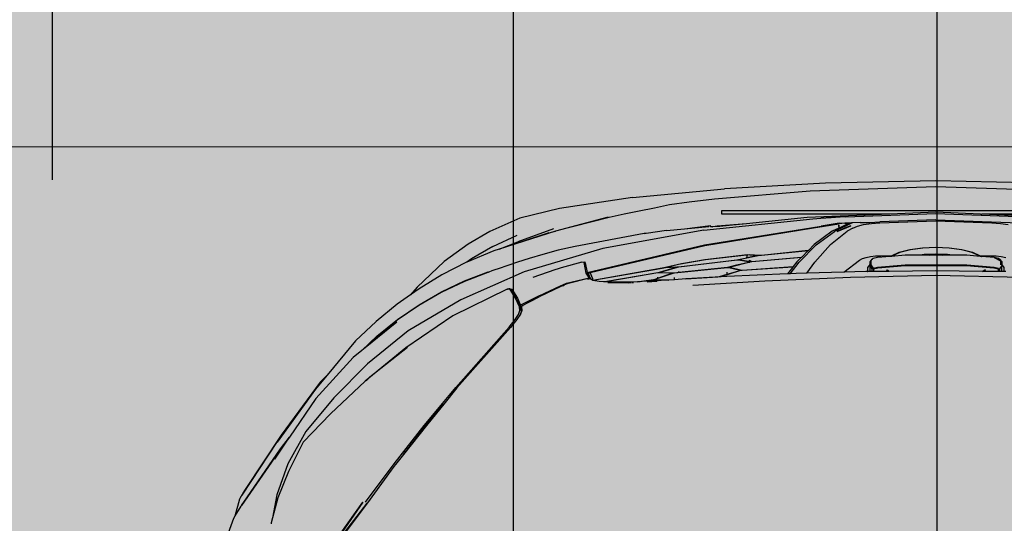
# Model space of a CAD drawing. Units: inches. Extents: x 1884 to 2398, y 474 to 1488.
# Tile 16 of 39: x 2186 to 2233, y 736 to 761. Entities that reach past the tile are written whole.
import ezdxf

# ---------------------------------------------------------------- set-up
doc = ezdxf.new("R2010")
doc.units = ezdxf.units.IN
doc.header["$MEASUREMENT"] = 0
doc.layers.get('0').update_dxf_attribs({"color": 250})
for name, color, linetype, lineweight in [('A-ANNO-DIMS', 2, 'Continuous', 18), ('A-FLOR-STRS', 7, 'Continuous', 20), ('C-VEHI', 8, 'Continuous', 18)]:
    doc.layers.add(name, color=color, linetype=linetype, lineweight=lineweight)
doc.layers.add('A-FLOR-STRS-PATT', color=251, linetype='Continuous', lineweight=13, true_color=0x636466)
doc.layers.add('L-PVMT-PATT', color=9, linetype='Continuous', lineweight=13, true_color=0xc7c8ca)
doc.layers.add('Edges', color=250, linetype='Continuous')
doc.styles.get("Standard").update_dxf_attribs({"font": 'arial.ttf'})
doc.dimstyles.get("Standard").update_dxf_attribs({"dimtxt": 7, "dimasz": 0.18, "dimexe": 0.18, "dimexo": 0.0625, "dimgap": 0.09, "dimtad": 0, "dimtih": 1, "dimtoh": 1, "dimzin": 0, "dimdsep": 46, "dimlunit": 3, "dimtxsty": 'Standard', "dimcen": 0.09, "dimadec": 0, "dimazin": 0, "dimtfac": 1, "dimtofl": 0, "dimtmove": 0, "dimatfit": 3, "dimfxl": 1, "dimtolj": 1, "dimtzin": 0, "dimarcsym": 0})

# ---------------------------------------------------------------- blocks, each defined once
blk = doc.blocks.new('Nissan Qashqai pl')
at = {"layer": 'Edges'}
for p, q in [((7.3216, 11.6621), (7.3216, 12.1821)), ((7.3261, 12.1821), (7.3261, 11.9779)), ((7.298, 12.075), (7.2928, 11.9221)), ((7.3302, 12.0785), (7.3261, 11.9779)), ((7.2884, 12.0562), (7.2857, 11.9221)), ((7.3251, 11.9221), (7.3291, 12.0316)), ((7.3329, 11.9221), (7.3365, 12.0237)), ((7.4002, 11.9221), (7.4025, 12.026)), ((7.3373, 12.0004), (7.3386, 12.01)), ((7.3775, 12.0015), (7.3786, 12.007)), ((7.3909, 12.0051), (7.387, 12.0021)), ((7.3956, 12.0051), (7.3909, 12.0051)), ((7.3959, 12.0049), (7.3956, 12.0051)), ((7.3959, 12.0051), (7.3956, 12.0051)), ((7.3959, 12.0049), (7.3958, 12.0018)), ((7.3959, 12.0071), (7.3959, 12.0051)), ((7.3959, 12.0051), (7.3959, 12.0049)), ((7.3367, 11.99), (7.3373, 12.0004)), ((7.3765, 11.989), (7.3768, 11.9954)), ((7.3768, 11.9954), (7.3775, 12.0015)), ((7.3787, 11.9928), (7.3774, 11.9778)), ((7.3798, 11.9983), (7.3787, 11.9928)), ((7.3787, 11.9928), (7.38, 11.9953)), ((7.3808, 11.9993), (7.3798, 11.9983)), ((7.3807, 11.9991), (7.3798, 11.9983)), ((7.38, 11.9953), (7.383, 12.0011)), ((7.3807, 11.9991), (7.3808, 11.9993)), ((7.381, 11.9993), (7.3807, 11.9991)), ((7.3808, 11.9993), (7.384, 12.0021)), ((7.381, 11.9993), (7.3808, 11.9993)), ((7.383, 12.0011), (7.381, 11.9993)), ((7.3866, 12.0011), (7.383, 12.0011)), ((7.384, 12.0021), (7.387, 12.0021)), ((7.3868, 12.002), (7.3866, 12.0011)), ((7.3875, 12.0011), (7.3866, 12.0011)), ((7.387, 12.0021), (7.3868, 12.002)), ((7.387, 12.0021), (7.3885, 12.0021)), ((7.3876, 11.9595), (7.3904, 11.9928)), ((7.3885, 12.0021), (7.3925, 11.9993)), ((7.3955, 12.0021), (7.3885, 12.0021)), ((7.3917, 11.9926), (7.3889, 11.9594)), ((7.3904, 11.9928), (7.3916, 11.9983)), ((7.3929, 11.9981), (7.3917, 11.9926)), ((7.3925, 11.9993), (7.3958, 11.9993)), ((7.3925, 11.9993), (7.3929, 11.9981)), ((7.3958, 11.9981), (7.3929, 11.9981)), ((7.3955, 12.0021), (7.3958, 12.0018)), ((7.3958, 11.9981), (7.3956, 11.9801)), ((7.3958, 12.0018), (7.3958, 11.9993)), ((7.3958, 11.9993), (7.3958, 11.9981)), ((7.3343, 11.9221), (7.3367, 11.99)), ((7.3761, 11.9751), (7.3765, 11.989)), ((7.3938, 11.9823), (7.3956, 11.9801)), ((7.3956, 11.9788), (7.3938, 11.981)), ((7.3956, 11.9788), (7.3951, 11.9221)), ((7.3956, 11.9801), (7.3956, 11.9788)), ((7.3261, 11.9764), (7.3238, 11.9221)), ((7.3261, 11.9764), (7.3261, 11.9779)), ((7.369, 11.9536), (7.3724, 11.9667)), ((7.3724, 11.9667), (7.3761, 11.9751)), ((7.3771, 11.9757), (7.3727, 11.9658)), ((7.3773, 11.9759), (7.3759, 11.9595)), ((7.3761, 11.9751), (7.3769, 11.9767)), ((7.3769, 11.9767), (7.3771, 11.977)), ((7.3774, 11.9778), (7.3771, 11.9771)), ((7.3771, 11.9771), (7.3774, 11.9774)), ((7.3771, 11.9771), (7.3771, 11.977)), ((7.3773, 11.9759), (7.3771, 11.9757)), ((7.3774, 11.9774), (7.3773, 11.9759)), ((7.3774, 11.9774), (7.3774, 11.9778)), ((7.3727, 11.9658), (7.3693, 11.953)), ((7.3759, 11.9595), (7.3759, 11.9417)), ((7.3876, 11.8847), (7.3876, 11.9595)), ((7.3889, 11.9594), (7.3889, 11.8848)), ((7.3668, 11.9384), (7.369, 11.9536)), ((7.3693, 11.953), (7.3672, 11.9381)), ((7.3661, 11.9221), (7.3668, 11.9384)), ((7.3672, 11.9381), (7.3665, 11.9221)), ((7.3751, 11.9363), (7.3745, 11.9221)), ((7.3759, 11.9417), (7.3751, 11.9363)), ((7.3759, 11.9417), (7.3759, 11.9303)), ((7.2857, 11.9221), (7.2884, 11.7879)), ((7.2928, 11.9221), (7.298, 11.7692)), ((7.3238, 11.9221), (7.3261, 11.8662)), ((7.3291, 11.8126), (7.3251, 11.9221)), ((7.3329, 11.9221), (7.3354, 11.8539)), ((7.3367, 11.8541), (7.3343, 11.9221)), ((7.3668, 11.9057), (7.3661, 11.9221)), ((7.3665, 11.9221), (7.3672, 11.9061)), ((7.3745, 11.9221), (7.3751, 11.9078)), ((7.3755, 11.9221), (7.3759, 11.9303)), ((7.3759, 11.9139), (7.3755, 11.9221)), ((7.3759, 11.9303), (7.3759, 11.9139)), ((7.3951, 11.9221), (7.3956, 11.8653)), ((7.4025, 11.8181), (7.4002, 11.9221)), ((7.3751, 11.9078), (7.3759, 11.9025)), ((7.3759, 11.9139), (7.3759, 11.9025)), ((7.369, 11.8905), (7.3668, 11.9057)), ((7.3672, 11.9061), (7.3693, 11.8911)), ((7.3759, 11.9025), (7.3759, 11.8847)), ((7.3724, 11.8775), (7.369, 11.8905)), ((7.3693, 11.8911), (7.3727, 11.8783)), ((7.3759, 11.8847), (7.3773, 11.8682)), ((7.3904, 11.8513), (7.3876, 11.8847)), ((7.3889, 11.8848), (7.3917, 11.8516)), ((7.3761, 11.8691), (7.3724, 11.8775)), ((7.3727, 11.8783), (7.3771, 11.8685)), ((7.3261, 11.8662), (7.3302, 11.7656)), ((7.3261, 11.8662), (7.3261, 11.6621)), ((7.3765, 11.8551), (7.3761, 11.8691)), ((7.3769, 11.8674), (7.3761, 11.8691)), ((7.3771, 11.8671), (7.3769, 11.8674)), ((7.3771, 11.8685), (7.3773, 11.8682)), ((7.3771, 11.8671), (7.3771, 11.8671)), ((7.3771, 11.8671), (7.3774, 11.8664)), ((7.3774, 11.8668), (7.3771, 11.8671)), ((7.3773, 11.8682), (7.3774, 11.8668)), ((7.3774, 11.8668), (7.3774, 11.8664)), ((7.3774, 11.8664), (7.3787, 11.8513)), ((7.3938, 11.8632), (7.3956, 11.8653)), ((7.3956, 11.864), (7.3938, 11.8619)), ((7.3956, 11.8653), (7.3956, 11.864)), ((7.3956, 11.864), (7.3958, 11.8461)), ((7.3361, 11.8416), (7.3354, 11.8539)), ((7.3373, 11.8438), (7.3367, 11.8541)), ((7.3768, 11.8488), (7.3765, 11.8551)), ((7.3775, 11.8427), (7.3768, 11.8488)), ((7.3787, 11.8513), (7.3798, 11.8459)), ((7.3916, 11.8459), (7.3904, 11.8513)), ((7.3917, 11.8516), (7.3929, 11.8461)), ((7.3362, 11.8301), (7.3361, 11.8416)), ((7.3386, 11.8342), (7.3373, 11.8438)), ((7.3786, 11.8372), (7.3775, 11.8427)), ((7.3801, 11.8327), (7.3786, 11.8372)), ((7.3798, 11.8459), (7.3808, 11.8448)), ((7.3808, 11.8448), (7.3807, 11.8451)), ((7.3808, 11.8448), (7.381, 11.8448)), ((7.384, 11.8421), (7.3808, 11.8448)), ((7.383, 11.8431), (7.3875, 11.8431)), ((7.387, 11.8421), (7.384, 11.8421)), ((7.387, 11.8421), (7.3909, 11.8391)), ((7.3885, 11.8421), (7.387, 11.8421)), ((7.3875, 11.8431), (7.3916, 11.8459)), ((7.3925, 11.8448), (7.3885, 11.8421)), ((7.3955, 11.8421), (7.3885, 11.8421)), ((7.3909, 11.8391), (7.3956, 11.8391)), ((7.3929, 11.8461), (7.3925, 11.8448)), ((7.3958, 11.8448), (7.3925, 11.8448)), ((7.3929, 11.8461), (7.3958, 11.8461)), ((7.3958, 11.8423), (7.3955, 11.8421)), ((7.3956, 11.8391), (7.3959, 11.8392)), ((7.3956, 11.8391), (7.3959, 11.8391)), ((7.3958, 11.8461), (7.3958, 11.8448)), ((7.3958, 11.8448), (7.3958, 11.8423)), ((7.3958, 11.8423), (7.3959, 11.8392)), ((7.3959, 11.8392), (7.3959, 11.8391)), ((7.3959, 11.8391), (7.3959, 11.8371)), ((7.3959, 11.8371), (7.3966, 11.8103)), ((7.3362, 11.8301), (7.3365, 11.8204)), ((7.3407, 11.8266), (7.3386, 11.8342)), ((7.3432, 11.821), (7.3407, 11.8266)), ((7.3818, 11.8291), (7.3801, 11.8327)), ((7.3966, 11.8103), (7.3818, 11.8291)), ((7.3291, 11.8126), (7.3294, 11.8057)), ((7.3362, 11.8194), (7.3365, 11.8204)), ((7.3367, 11.8196), (7.3362, 11.8194)), ((7.3365, 11.812), (7.3362, 11.8194)), ((7.3365, 11.8204), (7.3471, 11.7987)), ((7.3369, 11.8047), (7.3365, 11.812)), ((7.3369, 11.8155), (7.3374, 11.8165)), ((7.3369, 11.8113), (7.3369, 11.8155)), ((7.3369, 11.8155), (7.338, 11.8151)), ((7.3369, 11.8113), (7.3377, 11.8044)), ((7.3374, 11.8165), (7.338, 11.8151)), ((7.338, 11.8151), (7.343, 11.8045)), ((7.3401, 11.8186), (7.3431, 11.8112)), ((7.347, 11.8021), (7.3401, 11.8186)), ((7.3431, 11.8112), (7.347, 11.8021)), ((7.3432, 11.821), (7.3468, 11.8142)), ((7.363, 11.794), (7.3468, 11.8142)), ((7.4072, 11.7142), (7.4025, 11.8181)), ((7.3301, 11.7949), (7.3294, 11.8057)), ((7.3295, 11.8012), (7.3309, 11.7822)), ((7.3295, 11.8012), (7.3301, 11.7949)), ((7.3369, 11.8047), (7.3405, 11.7825)), ((7.3377, 11.8042), (7.3377, 11.8044)), ((7.341, 11.7837), (7.3377, 11.8042)), ((7.343, 11.8045), (7.3396, 11.8043)), ((7.3396, 11.8043), (7.3431, 11.8042)), ((7.343, 11.8045), (7.3431, 11.8042)), ((7.3431, 11.8042), (7.3469, 11.7961)), ((7.3966, 11.8103), (7.3978, 11.7651)), ((7.2884, 11.7879), (7.2951, 11.6651)), ((7.3309, 11.7822), (7.3301, 11.7949)), ((7.3469, 11.7961), (7.3631, 11.774)), ((7.3633, 11.7767), (7.3471, 11.7987)), ((7.3842, 11.7749), (7.363, 11.794)), ((7.3317, 11.7724), (7.3309, 11.7822)), ((7.3635, 11.6409), (7.3405, 11.7825)), ((7.3426, 11.7735), (7.341, 11.7837)), ((7.3845, 11.7558), (7.3633, 11.7767)), ((7.298, 11.7692), (7.3078, 11.6532)), ((7.3302, 11.7656), (7.3378, 11.6921)), ((7.3455, 11.64), (7.3317, 11.7724)), ((7.364, 11.6413), (7.3426, 11.7735)), ((7.3631, 11.774), (7.3701, 11.7671)), ((7.3759, 11.7101), (7.3701, 11.7671)), ((7.3701, 11.7671), (7.3704, 11.7668)), ((7.3704, 11.7668), (7.3761, 11.71)), ((7.3704, 11.7668), (7.3783, 11.759)), ((7.3978, 11.7651), (7.3842, 11.7749)), ((7.3978, 11.7651), (7.3982, 11.7521)), ((7.3836, 11.6983), (7.3783, 11.759)), ((7.3783, 11.759), (7.3788, 11.7585)), ((7.3788, 11.7585), (7.384, 11.6982)), ((7.3788, 11.7585), (7.3841, 11.7532)), ((7.3841, 11.7532), (7.3896, 11.7488)), ((7.3985, 11.7448), (7.3845, 11.7558)), ((7.3982, 11.7521), (7.3985, 11.7448)), ((7.3941, 11.6865), (7.3896, 11.7488)), ((7.3896, 11.7488), (7.3903, 11.7483)), ((7.3903, 11.7483), (7.3945, 11.6865)), ((7.3903, 11.7483), (7.3986, 11.7417)), ((7.3985, 11.7448), (7.3986, 11.7417)), ((7.3986, 11.7417), (7.4018, 11.6678)), ((7.375, 11.6957), (7.376, 11.7081)), ((7.3762, 11.7062), (7.3757, 11.6959)), ((7.376, 11.7081), (7.3759, 11.7101)), ((7.3761, 11.71), (7.3763, 11.7081)), ((7.3762, 11.7062), (7.3764, 11.7061)), ((7.3763, 11.7081), (7.3813, 11.6842)), ((7.3764, 11.7061), (7.3792, 11.6924)), ((7.4124, 11.6265), (7.4072, 11.7142)), ((7.3378, 11.6921), (7.3407, 11.6563)), ((7.3378, 11.6921), (7.34, 11.671)), ((7.3813, 11.642), (7.375, 11.6957)), ((7.3757, 11.6959), (7.3756, 11.6933)), ((7.3792, 11.6924), (7.3756, 11.6933)), ((7.3756, 11.6933), (7.3815, 11.6413)), ((7.3757, 11.6959), (7.3757, 11.6959)), ((7.3812, 11.6823), (7.3792, 11.6924)), ((7.3817, 11.6844), (7.3832, 11.6949)), ((7.3838, 11.6944), (7.382, 11.6823)), ((7.3824, 11.6955), (7.3836, 11.6983)), ((7.3835, 11.6973), (7.3824, 11.6955)), ((7.3834, 11.6959), (7.3824, 11.6955)), ((7.3824, 11.6955), (7.3832, 11.6949)), ((7.3832, 11.695), (7.3824, 11.6955)), ((7.3832, 11.695), (7.3834, 11.6959)), ((7.3838, 11.6947), (7.3832, 11.695)), ((7.3832, 11.6949), (7.3838, 11.6944)), ((7.3837, 11.696), (7.3834, 11.6959)), ((7.3835, 11.6973), (7.3836, 11.6983)), ((7.3836, 11.6975), (7.3835, 11.6973)), ((7.3836, 11.6975), (7.3836, 11.6983)), ((7.384, 11.6982), (7.3836, 11.6975)), ((7.3844, 11.6963), (7.3837, 11.696)), ((7.3838, 11.6947), (7.3837, 11.696)), ((7.3843, 11.6944), (7.3838, 11.6947)), ((7.3843, 11.6942), (7.3838, 11.6944)), ((7.3843, 11.6944), (7.3844, 11.6963)), ((7.3843, 11.6942), (7.3843, 11.6944)), ((7.3877, 11.6803), (7.3843, 11.6942)), ((7.3844, 11.6963), (7.3903, 11.6725)), ((7.3815, 11.6804), (7.3812, 11.6823)), ((7.3813, 11.6842), (7.3817, 11.6844)), ((7.3817, 11.6841), (7.3813, 11.6842)), ((7.3899, 11.6094), (7.3815, 11.6804)), ((7.3817, 11.6841), (7.3817, 11.6844)), ((7.382, 11.6823), (7.382, 11.6803)), ((7.382, 11.6803), (7.3903, 11.6095)), ((7.3874, 11.6803), (7.3877, 11.6803)), ((7.3901, 11.6707), (7.3877, 11.6803)), ((7.3909, 11.6728), (7.3939, 11.6846)), ((7.3943, 11.6827), (7.3913, 11.6705)), ((7.3939, 11.6846), (7.3941, 11.6865)), ((7.3943, 11.6827), (7.3949, 11.6826)), ((7.3943, 11.6827), (7.395, 11.6825)), ((7.3945, 11.6865), (7.3951, 11.6835)), ((7.395, 11.6825), (7.3949, 11.6826)), ((7.399, 11.6686), (7.395, 11.6825)), ((7.3951, 11.6835), (7.4021, 11.6609)), ((7.34, 11.671), (7.341, 11.6594)), ((7.3905, 11.6687), (7.3901, 11.6707)), ((7.3909, 11.6728), (7.3903, 11.6725)), ((7.3909, 11.6725), (7.3903, 11.6725)), ((7.3966, 11.6095), (7.3905, 11.6687)), ((7.3909, 11.6725), (7.3909, 11.6728)), ((7.3913, 11.6705), (7.3911, 11.6687)), ((7.3911, 11.6687), (7.3977, 11.6042)), ((7.399, 11.6686), (7.3967, 11.6686)), ((7.4017, 11.6592), (7.399, 11.6686)), ((7.4018, 11.6678), (7.4022, 11.6609)), ((7.3059, 11.5532), (7.2951, 11.6651)), ((7.3261, 11.6621), (7.3216, 11.6621)), ((7.3407, 11.6563), (7.3413, 11.6509)), ((7.341, 11.6594), (7.3413, 11.6511)), ((7.4022, 11.6571), (7.4017, 11.6592)), ((7.4022, 11.6609), (7.4021, 11.6609)), ((7.4022, 11.6609), (7.4021, 11.6609)), ((7.4022, 11.6609), (7.4048, 11.618)), ((7.4022, 11.6609), (7.4022, 11.6609)), ((7.4048, 11.618), (7.4022, 11.6571)), ((7.3078, 11.6532), (7.3113, 11.6224)), ((7.3401, 11.648), (7.34, 11.648)), ((7.3438, 11.6167), (7.34, 11.648)), ((7.341, 11.648), (7.3401, 11.648)), ((7.341, 11.648), (7.3413, 11.6509)), ((7.3414, 11.648), (7.341, 11.648)), ((7.341, 11.648), (7.3414, 11.648)), ((7.3438, 11.6167), (7.3412, 11.646)), ((7.3413, 11.6511), (7.3413, 11.6509)), ((7.3413, 11.6509), (7.3415, 11.6488)), ((7.3455, 11.64), (7.3676, 11.5172)), ((7.3971, 11.4981), (7.3635, 11.6409)), ((7.3968, 11.5018), (7.364, 11.6413)), ((7.3869, 11.6094), (7.3813, 11.642)), ((7.3815, 11.6413), (7.3864, 11.6131)), ((7.3113, 11.6224), (7.3149, 11.5984)), ((7.3457, 11.5947), (7.3438, 11.6167)), ((7.3864, 11.6131), (7.3909, 11.5933)), ((7.3912, 11.5914), (7.3869, 11.6094)), ((7.3901, 11.6073), (7.3899, 11.6094)), ((7.3903, 11.6095), (7.3908, 11.6076)), ((7.3908, 11.6076), (7.3965, 11.5881)), ((7.3966, 11.6095), (7.3957, 11.6095)), ((7.3972, 11.6042), (7.3966, 11.6095)), ((7.4048, 11.618), (7.4057, 11.6042)), ((7.3149, 11.5984), (7.3186, 11.58)), ((7.391, 11.5935), (7.3901, 11.6073)), ((7.3906, 11.6055), (7.391, 11.6055)), ((7.3906, 11.6055), (7.391, 11.6054)), ((7.3906, 11.6055), (7.3914, 11.5914)), ((7.391, 11.6054), (7.391, 11.6055)), ((7.3967, 11.5862), (7.391, 11.6054)), ((7.3968, 11.5882), (7.3972, 11.6021)), ((7.3972, 11.6021), (7.3972, 11.6042)), ((7.3977, 11.6003), (7.3973, 11.5862)), ((7.3977, 11.6042), (7.3982, 11.6022)), ((7.3977, 11.6003), (7.3983, 11.6002)), ((7.3977, 11.6003), (7.3983, 11.6001)), ((7.3982, 11.6022), (7.4048, 11.5829)), ((7.3983, 11.6001), (7.3983, 11.6002)), ((7.4038, 11.5843), (7.3983, 11.6001)), ((7.4057, 11.6042), (7.4032, 11.6042)), ((7.4053, 11.5831), (7.4061, 11.5969)), ((7.4057, 11.6042), (7.4061, 11.597)), ((7.4061, 11.5969), (7.4061, 11.597)), ((7.4061, 11.5969), (7.4064, 11.5919)), ((7.3457, 11.5947), (7.3494, 11.57)), ((7.391, 11.5935), (7.3909, 11.5933)), ((7.391, 11.5934), (7.3909, 11.5933)), ((7.3916, 11.5894), (7.3912, 11.5914)), ((7.3914, 11.5914), (7.3917, 11.5895)), ((7.4062, 11.5053), (7.3916, 11.5894)), ((7.3917, 11.5895), (7.4065, 11.505)), ((7.3968, 11.5882), (7.3965, 11.5881)), ((7.3971, 11.5842), (7.3967, 11.5862)), ((7.3968, 11.5882), (7.3973, 11.5884)), ((7.4083, 11.5184), (7.3971, 11.5842)), ((7.3973, 11.5862), (7.3975, 11.5843)), ((7.3975, 11.5843), (7.4084, 11.5198)), ((7.4038, 11.5843), (7.4028, 11.5843)), ((7.4049, 11.5811), (7.4038, 11.5843)), ((7.4064, 11.5919), (7.406, 11.5834)), ((7.4064, 11.5919), (7.4069, 11.5844)), ((7.4069, 11.5844), (7.4079, 11.5644)), ((7.3186, 11.58), (7.3223, 11.5616)), ((7.4053, 11.5831), (7.4048, 11.5829)), ((7.4053, 11.583), (7.4048, 11.5829)), ((7.4054, 11.5791), (7.4049, 11.5811)), ((7.406, 11.5834), (7.4053, 11.5831)), ((7.406, 11.5833), (7.4053, 11.583)), ((7.4053, 11.583), (7.4053, 11.5831)), ((7.4081, 11.5593), (7.4054, 11.5791)), ((7.406, 11.5833), (7.4058, 11.581)), ((7.4058, 11.581), (7.4059, 11.579)), ((7.4059, 11.579), (7.4079, 11.5644)), ((7.406, 11.5834), (7.406, 11.5833)), ((7.4081, 11.5711), (7.4075, 11.5828)), ((7.3223, 11.5616), (7.3261, 11.5433)), ((7.3494, 11.57), (7.3497, 11.5674)), ((7.3494, 11.57), (7.3498, 11.5674)), ((7.3497, 11.5674), (7.3653, 11.4838)), ((7.4079, 11.5644), (7.4081, 11.5604)), ((7.4079, 11.5644), (7.4081, 11.5629)), ((7.4081, 11.5604), (7.4081, 11.5593)), ((7.3059, 11.5532), (7.3193, 11.4645)), ((7.4081, 11.5593), (7.4087, 11.5405)), ((7.4092, 11.5416), (7.409, 11.5485)), ((7.4096, 11.549), (7.4092, 11.5521)), ((7.4093, 11.5546), (7.4095, 11.5529)), ((7.3261, 11.5433), (7.33, 11.5249)), ((7.4087, 11.5405), (7.4087, 11.5246)), ((7.4092, 11.5258), (7.4092, 11.5416)), ((7.3297, 11.5237), (7.3467, 11.4596)), ((7.33, 11.5249), (7.3467, 11.4596)), ((7.4087, 11.5246), (7.4084, 11.5198)), ((7.4091, 11.5235), (7.4092, 11.5258)), ((7.3676, 11.5172), (7.3963, 11.4215)), ((7.408, 11.5129), (7.4066, 11.5052)), ((7.4083, 11.5184), (7.408, 11.5129)), ((7.4084, 11.5198), (7.4083, 11.5184)), ((7.4046, 11.5053), (7.3968, 11.5018)), ((7.398, 11.4993), (7.3968, 11.5018)), ((7.4026, 11.5002), (7.3976, 11.4971)), ((7.398, 11.4993), (7.4048, 11.5024)), ((7.4012, 11.5001), (7.398, 11.4993)), ((7.3983, 11.4983), (7.4012, 11.5001)), ((7.4012, 11.5001), (7.4033, 11.5014)), ((7.403, 11.5005), (7.4026, 11.5002)), ((7.403, 11.5005), (7.4028, 11.5004)), ((7.4033, 11.5007), (7.403, 11.5005)), ((7.4033, 11.5014), (7.4042, 11.502)), ((7.4042, 11.502), (7.4033, 11.5007)), ((7.4033, 11.5005), (7.4033, 11.5007)), ((7.4034, 11.5005), (7.4033, 11.5005)), ((7.4101, 11.4733), (7.4033, 11.5005)), ((7.4043, 11.5016), (7.404, 11.5012)), ((7.4043, 11.5014), (7.404, 11.5012)), ((7.404, 11.5012), (7.4108, 11.4738)), ((7.4042, 11.502), (7.4044, 11.502)), ((7.4043, 11.5016), (7.4042, 11.502)), ((7.4044, 11.502), (7.4043, 11.5016)), ((7.4046, 11.5016), (7.4043, 11.5014)), ((7.4043, 11.5014), (7.4043, 11.5016)), ((7.4045, 11.5008), (7.4043, 11.5014)), ((7.4046, 11.5023), (7.4044, 11.502)), ((7.4044, 11.502), (7.4046, 11.502)), ((7.4048, 11.5008), (7.4045, 11.5008)), ((7.405, 11.4985), (7.4045, 11.5008)), ((7.4062, 11.5053), (7.4046, 11.5053)), ((7.4046, 11.5023), (7.4048, 11.5024)), ((7.405, 11.5023), (7.4046, 11.5023)), ((7.4046, 11.5023), (7.4046, 11.502)), ((7.4046, 11.502), (7.4047, 11.5018)), ((7.4046, 11.502), (7.4048, 11.502)), ((7.4047, 11.5018), (7.4046, 11.5016)), ((7.4048, 11.502), (7.4047, 11.5018)), ((7.4048, 11.5024), (7.4052, 11.5027)), ((7.4052, 11.5026), (7.4048, 11.5024)), ((7.405, 11.5023), (7.4048, 11.502)), ((7.4052, 11.5026), (7.405, 11.5023)), ((7.4063, 11.5047), (7.4052, 11.5027)), ((7.4052, 11.5027), (7.4052, 11.5026)), ((7.4063, 11.5047), (7.4062, 11.5053)), ((7.4065, 11.505), (7.4063, 11.5047)), ((7.4066, 11.5052), (7.4065, 11.505)), ((7.3853, 11.4958), (7.3841, 11.4956)), ((7.3844, 11.4916), (7.3841, 11.4956)), ((7.3846, 11.4946), (7.3844, 11.4916)), ((7.3844, 11.4916), (7.3914, 11.4667)), ((7.3976, 11.4971), (7.3846, 11.4946)), ((7.3853, 11.4958), (7.3846, 11.4946)), ((7.3853, 11.4958), (7.3971, 11.4981)), ((7.3971, 11.4981), (7.3983, 11.4983)), ((7.3653, 11.4838), (7.3699, 11.4629)), ((7.3193, 11.4645), (7.3309, 11.4166)), ((7.3914, 11.4667), (7.3925, 11.4629)), ((7.4115, 11.4695), (7.4101, 11.4733)), ((7.4108, 11.4738), (7.4122, 11.47)), ((7.4131, 11.4659), (7.4115, 11.4695)), ((7.4122, 11.47), (7.4139, 11.4664)), ((7.4126, 11.47), (7.4125, 11.4702)), ((7.4132, 11.4685), (7.4126, 11.47)), ((7.4255, 11.4398), (7.4131, 11.4659)), ((7.4139, 11.4664), (7.4267, 11.4401)), ((7.344, 11.4572), (7.3596, 11.4139)), ((7.3489, 11.4517), (7.3467, 11.4596)), ((7.3467, 11.4596), (7.3686, 11.3913)), ((7.3699, 11.4629), (7.375, 11.4442)), ((7.3925, 11.4629), (7.3937, 11.4591)), ((7.3937, 11.4591), (7.4029, 11.4321)), ((7.3489, 11.4517), (7.3686, 11.3913)), ((7.375, 11.4442), (7.3799, 11.4278)), ((7.4379, 11.4179), (7.4267, 11.4401)), ((7.4255, 11.4398), (7.4367, 11.4174)), ((7.3309, 11.4166), (7.347, 11.3798)), ((7.3799, 11.4278), (7.3845, 11.4136)), ((7.3963, 11.4215), (7.4302, 11.3449)), ((7.4387, 11.4162), (7.4282, 11.4113)), ((7.4283, 11.4135), (7.4359, 11.417)), ((7.4296, 11.4129), (7.4383, 11.417)), ((7.4359, 11.417), (7.4367, 11.4174)), ((7.4383, 11.417), (7.4367, 11.4174)), ((7.4375, 11.42), (7.4384, 11.4182)), ((7.4379, 11.4179), (7.4384, 11.4182)), ((7.4389, 11.4173), (7.4379, 11.4179)), ((7.4383, 11.417), (7.4379, 11.4179)), ((7.4389, 11.4173), (7.4383, 11.417)), ((7.4384, 11.4182), (7.4387, 11.4183)), ((7.4387, 11.4183), (7.443, 11.4188)), ((7.4431, 11.4166), (7.4387, 11.4162)), ((7.4389, 11.4173), (7.44, 11.4178)), ((7.4442, 11.4183), (7.44, 11.4178)), ((7.443, 11.4188), (7.4477, 11.4172)), ((7.4479, 11.4149), (7.4431, 11.4166)), ((7.4477, 11.4172), (7.4442, 11.4183)), ((7.4477, 11.4172), (7.4541, 11.4128)), ((7.3655, 11.3837), (7.3514, 11.4133)), ((7.3686, 11.3913), (7.3596, 11.4139)), ((7.3845, 11.4136), (7.3925, 11.3899)), ((7.4167, 11.4049), (7.417, 11.4065)), ((7.4172, 11.4047), (7.4167, 11.4049)), ((7.4169, 11.4036), (7.4167, 11.4049)), ((7.4282, 11.4113), (7.4169, 11.4044)), ((7.4172, 11.4047), (7.4169, 11.4044)), ((7.4169, 11.4044), (7.4169, 11.4036)), ((7.417, 11.4065), (7.4283, 11.4135)), ((7.4183, 11.406), (7.4172, 11.4047)), ((7.4296, 11.4129), (7.4183, 11.406)), ((7.4541, 11.4108), (7.4479, 11.4149)), ((7.4541, 11.4128), (7.4638, 11.4051)), ((7.4635, 11.4034), (7.4541, 11.4108)), ((7.4638, 11.4051), (7.5371, 11.34)), ((7.4172, 11.4018), (7.4169, 11.4036)), ((7.4169, 11.4036), (7.4169, 11.403)), ((7.4169, 11.403), (7.4172, 11.4011)), ((7.4174, 11.4013), (7.4172, 11.4018)), ((7.4172, 11.4011), (7.4498, 11.3349)), ((7.4174, 11.4013), (7.4175, 11.4012)), ((7.5369, 11.3385), (7.4635, 11.4034)), ((7.3655, 11.3837), (7.3805, 11.3576)), ((7.3686, 11.3913), (7.3707, 11.3849)), ((7.3707, 11.3849), (7.3843, 11.3522)), ((7.3925, 11.3899), (7.3938, 11.3859)), ((7.3938, 11.3859), (7.3951, 11.3822)), ((7.3951, 11.3822), (7.3965, 11.3787)), ((7.347, 11.3798), (7.3624, 11.3535)), ((7.3962, 11.3781), (7.3965, 11.3787)), ((7.4071, 11.3493), (7.3962, 11.3781)), ((7.3965, 11.3787), (7.3969, 11.3777)), ((7.3969, 11.3777), (7.4078, 11.349)), ((7.3805, 11.3576), (7.3843, 11.3522)), ((7.3624, 11.3535), (7.3837, 11.3245)), ((7.3843, 11.3522), (7.3845, 11.3517)), ((7.3845, 11.3517), (7.3997, 11.3215)), ((7.4205, 11.3212), (7.4071, 11.3493)), ((7.4078, 11.349), (7.4211, 11.321)), ((7.4302, 11.3449), (7.4679, 11.2807)), ((7.4498, 11.3349), (7.4884, 11.2778)), ((7.5827, 11.3001), (7.5369, 11.3385)), ((7.5371, 11.34), (7.5568, 11.324)), ((7.3837, 11.3245), (7.4147, 11.2918)), ((7.3997, 11.3215), (7.4166, 11.2939)), ((7.4363, 11.294), (7.4205, 11.3212)), ((7.4211, 11.321), (7.4369, 11.2938)), ((7.584, 11.3013), (7.5568, 11.324)), ((7.5568, 11.324), (7.5829, 11.303)), ((7.6296, 11.2639), (7.5827, 11.3001)), ((7.5829, 11.303), (7.618, 11.275)), ((7.618, 11.275), (7.584, 11.3013)), ((7.4147, 11.2918), (7.4239, 11.2837)), ((7.4166, 11.2939), (7.4239, 11.2837)), ((7.4542, 11.2677), (7.4363, 11.294)), ((7.4369, 11.2938), (7.4549, 11.2675)), ((7.4239, 11.2837), (7.4354, 11.2675)), ((7.4679, 11.2807), (7.5081, 11.2311)), ((7.4882, 11.2797), (7.5243, 11.2341)), ((7.4884, 11.2778), (7.5289, 11.2283)), ((7.618, 11.275), (7.6301, 11.2654)), ((7.4354, 11.2675), (7.4565, 11.2419)), ((7.4744, 11.2427), (7.4542, 11.2677)), ((7.4549, 11.2675), (7.475, 11.2426)), ((7.4574, 11.267), (7.4885, 11.2283)), ((7.676, 11.2289), (7.6296, 11.2639)), ((7.6301, 11.2654), (7.6306, 11.2651)), ((7.6306, 11.2651), (7.6306, 11.265)), ((7.6306, 11.265), (7.6373, 11.2601)), ((7.6373, 11.2601), (7.6769, 11.2312)), ((7.4565, 11.2419), (7.4801, 11.2168)), ((7.4918, 11.2242), (7.4744, 11.2427)), ((7.475, 11.2426), (7.477, 11.2404)), ((7.477, 11.2404), (7.4765, 11.2411)), ((7.477, 11.2405), (7.4775, 11.2399)), ((7.4784, 11.2388), (7.477, 11.2404)), ((7.477, 11.2404), (7.4775, 11.2399)), ((7.4775, 11.2399), (7.4787, 11.2385)), ((7.4775, 11.2399), (7.4787, 11.2387)), ((7.4787, 11.2387), (7.4782, 11.2392)), ((7.4795, 11.2377), (7.4787, 11.2387)), ((7.4787, 11.2387), (7.4885, 11.2283)), ((7.4885, 11.2283), (7.4918, 11.2242)), ((7.5081, 11.2311), (7.5492, 11.1902)), ((7.5243, 11.2341), (7.5286, 11.2296)), ((7.5289, 11.2283), (7.5687, 11.1862)), ((7.7261, 11.1898), (7.6762, 11.2256)), ((7.6762, 11.2256), (7.7233, 11.1928)), ((7.6769, 11.2312), (7.7194, 11.1992)), ((7.7232, 11.1955), (7.6771, 11.2307)), ((7.4801, 11.2168), (7.5217, 11.1823)), ((7.4918, 11.2242), (7.5001, 11.2139)), ((7.5001, 11.2139), (7.5501, 11.1684)), ((7.5492, 11.1902), (7.59, 11.1565)), ((7.5304, 11.1737), (7.5217, 11.1823)), ((7.5217, 11.1823), (7.5387, 11.1682)), ((7.5687, 11.1862), (7.6032, 11.1533)), ((7.5304, 11.1737), (7.5946, 11.1262)), ((7.5387, 11.1682), (7.6031, 11.1217)), ((7.5501, 11.1684), (7.5969, 11.1365)), ((7.59, 11.1565), (7.6295, 11.1344)), ((7.6032, 11.1533), (7.6386, 11.1353)), ((7.6113, 11.1256), (7.5969, 11.1365)), ((7.5969, 11.1365), (7.6021, 11.1329)), ((7.6021, 11.1329), (7.6118, 11.1255)), ((7.6021, 11.1329), (7.6237, 11.1181)), ((7.6295, 11.1344), (7.667, 11.1212)), ((7.6386, 11.1353), (7.6708, 11.1225)), ((7.5946, 11.1262), (7.6608, 11.0825)), ((7.6676, 11.0791), (7.6024, 11.1221)), ((7.6759, 11.0809), (7.6113, 11.1256)), ((7.6118, 11.1255), (7.6799, 11.0783)), ((7.667, 11.1212), (7.6949, 11.1158)), ((7.6708, 11.1225), (7.6949, 11.1158)), ((7.6949, 11.1158), (7.701, 11.1141)), ((7.701, 11.1141), (7.7024, 11.1141)), ((7.6712, 11.0767), (7.6608, 11.0825)), ((7.6793, 11.0784), (7.6759, 11.0809)), ((7.6721, 11.0762), (7.6712, 11.0767)), ((7.6926, 11.0705), (7.6721, 11.0762)), ((7.6802, 11.0782), (7.6793, 11.0784)), ((7.6802, 11.0782), (7.6799, 11.0783)), ((7.6809, 11.0777), (7.6802, 11.0782)), ((7.6926, 11.0705), (7.6809, 11.0777)), ((7.6953, 11.0688), (7.6926, 11.0705)), ((7.7223, 11.059), (7.6953, 11.0688))]:
    blk.add_line(p, q, dxfattribs=at)
blk = doc.blocks.new('car')
blk.add_blockref('Nissan Qashqai pl', (-9.7433, -11.9151))
blk = doc.blocks.new('carr')
blk.add_blockref('car', (0.5124, -0.007))
blk = doc.blocks.new('*D24')
at = {"layer": 'A-ANNO-DIMS', "color": 0, "lineweight": -2, "transparency": 16777216}
for p, q in [((2187.713, 752.874), (2187.713, 778.861)), ((2272.242, 752.874), (2272.242, 778.861)), ((2187.893, 778.681), (2200.426, 778.681)), ((2272.062, 778.681), (2259.528, 778.681))]:
    blk.add_line(p, q, dxfattribs=at)
at = {"layer": 'A-ANNO-DIMS', "color": 0, "lineweight": 100, "transparency": 16777216}
for points in [[(2187.893, 778.711), (2187.893, 778.651), (2187.713, 778.681)], [(2272.062, 778.711), (2272.062, 778.651), (2272.242, 778.681)]]:
    blk.add_solid(points, dxfattribs=at)
at = {"layer": 'Defpoints', "color": 0, "lineweight": 100, "transparency": 16777216}
for p in [(2272.242, 778.681), (2187.713, 752.812), (2272.242, 752.812)]:
    blk.add_point(p, dxfattribs=at)
at = {"layer": 'A-ANNO-DIMS', "color": 0, "transparency": 16777216, "insert": (2229.977, 778.681), "char_height": 7, "attachment_point": 5}
blk.add_mtext('\\A1;7\'-0 1/2" TYP.', dxfattribs=at)
blk = doc.blocks.new('*D44')
at = {"layer": 'A-ANNO-DIMS', "color": 0, "lineweight": -2, "transparency": 16777216}
for p, q in [((2209.755, 1247.822), (2209.755, 484.005)), ((2230.029, 1247.822), (2230.029, 484.005)), ((2209.935, 484.185), (2229.849, 484.185)), ((2230.029, 484.185), (2230.209, 484.185))]:
    blk.add_line(p, q, dxfattribs=at)
at = {"layer": 'A-ANNO-DIMS', "color": 0, "lineweight": 100, "transparency": 16777216}
for points in [[(2209.935, 484.215), (2209.935, 484.155), (2209.755, 484.185)], [(2229.849, 484.215), (2229.849, 484.155), (2230.029, 484.185)]]:
    blk.add_solid(points, dxfattribs=at)
at = {"layer": 'Defpoints', "color": 0, "lineweight": 100, "transparency": 16777216}
for p in [(2209.755, 1247.885), (2230.029, 1247.885), (2230.029, 484.185)]:
    blk.add_point(p, dxfattribs=at)
at = {"layer": 'A-ANNO-DIMS', "color": 0, "transparency": 16777216, "insert": (2247.429, 484.185), "char_height": 7, "attachment_point": 5}
blk.add_mtext('\\A1;1\'-8 1/2"', dxfattribs=at)

msp = doc.modelspace()

# ---------------------------------------------------------------- hatches: boundary and pattern name
at = {"layer": 'A-FLOR-STRS-PATT'}
h = msp.add_hatch(color=256, dxfattribs=at)
h.dxf.hatch_style = 1
h.paths.add_polyline_path([(2238.447, 769.966), (2198.529, 769.966), (2193.526, 769.966), (2132.515, 769.966), (2126.529, 769.966), (2126.529, 762.15), (2238.447, 762.15)])
h.paths.add_polyline_path([(2238.447, 762.15), (2126.529, 762.15), (2126.529, 754.445), (2238.447, 754.445)])
at = {"layer": 'L-PVMT-PATT'}
h = msp.add_hatch(color=256, dxfattribs=at)
h.dxf.hatch_style = 1
h.paths.add_polyline_path([(2387.529, 769.966), (2351.529, 769.966), (2238.447, 769.966), (2238.447, 762.15), (2238.447, 754.445), (2126.529, 754.445), (2126.529, 676.183), (2134.868, 676.183), (2142.673, 676.183), (2142.673, 646.578), (2134.868, 646.578), (2126.529, 646.578), (2126.529, 640.17), (2387.529, 640.17)])
h.paths.add_polyline_path([(2387.529, 631.385), (2303.086, 631.385), (2303.086, 615.671), (2387.529, 615.671)])
h.paths.add_polyline_path([(2387.529, 640.17), (2126.529, 640.17), (2126.529, 631.385), (2387.529, 631.385)])
h.paths.add_polyline_path([(2393.529, 604.13), (2387.529, 604.13), (2387.529, 615.671), (2303.086, 615.671), (2303.086, 607.943), (2249.649, 607.943), (2126.529, 607.943), (2126.529, 533.885), (2393.529, 533.885)])
h.paths.add_polyline_path([(2257.825, 611.008), (2257.83, 611.337), (2257.915, 616.493), (2258.021, 621.805), (2258.146, 627.274), (2258.252, 631.385), (2126.529, 631.385), (2126.529, 611.008)])
h.paths.add_polyline_path([(2258.892, 611.285), (2258.888, 611.008), (2300.247, 611.008), (2300.247, 631.385), (2259.314, 631.385), (2259.206, 627.173), (2259.081, 621.72), (2258.976, 616.424)])

# ---------------------------------------------------------------- linework, layer by layer
at = {"layer": 'A-FLOR-STRS'}
msp.add_line((2126.529, 754.445), (2238.447, 754.445), dxfattribs=at)

# ---------------------------------------------------------------- block references
at = {"layer": 'C-VEHI', "xscale": 39.37007874015748, "yscale": 39.37007874015748, "zscale": 39.37007874015748, "rotation": 270}
msp.add_blockref('carr', (2229.977, 676.232), dxfattribs=at)

# ---------------------------------------------------------------- dimensions: what is measured, and where the dimension line sits
at = {"layer": 'A-ANNO-DIMS'}
dim = msp.add_linear_dim(base=(2230.029, 484.185), p1=(2209.755, 1247.885), p2=(2230.029, 1247.885), dimstyle='Standard', override={"dimdec": 1, "dimlfac": 1, "dimrnd": 0, "dimzin": 1, "dimdsep": 46, "dimlunit": 4, "dimfrac": 2}, dxfattribs=at)
dim.commit()
dim.dimension.update_dxf_attribs({"geometry": '*D44', "text_midpoint": (2247.429, 484.185)})
dim = msp.add_linear_dim(base=(2272.242, 778.681), p1=(2187.713, 752.812), p2=(2272.242, 752.812), text='<> TYP.', dimstyle='Standard', override={"dimdec": 1, "dimlfac": 1, "dimrnd": 0, "dimzin": 1, "dimdsep": 46, "dimlunit": 4, "dimfrac": 2}, dxfattribs=at)
dim.commit()
dim.dimension.update_dxf_attribs({"geometry": '*D24', "text_midpoint": (2229.977, 778.681)})

doc.saveas('drawing.dxf')
